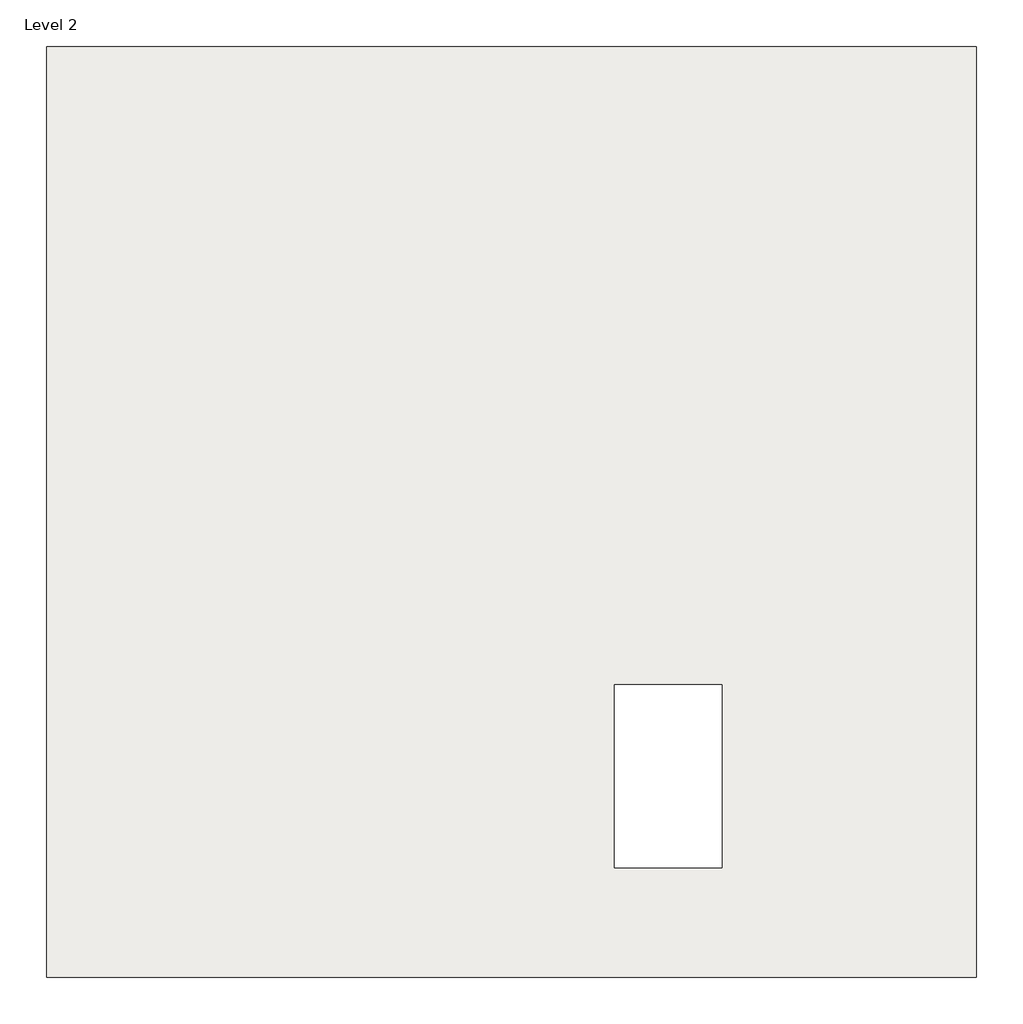
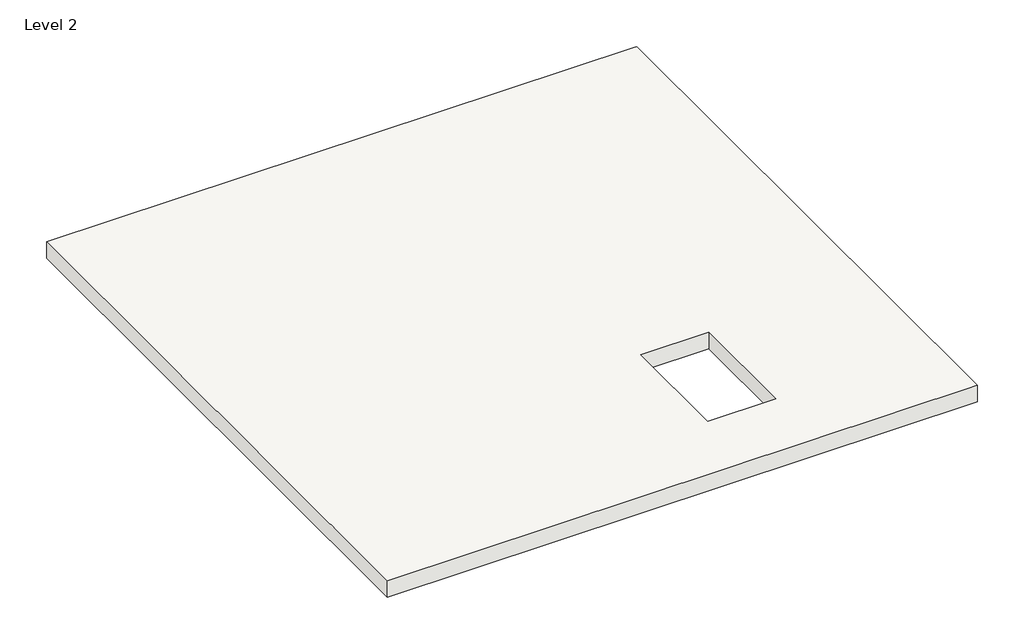
# One storey: 1 roof.
"""IFC4 building model written with IfcOpenShell, lengths in millimetres."""

from ifc_helpers import new_model, si_unit, frame, origin, place, context, project, spatial, polyline, outline, extrude, element, save

model = new_model("IFC4")

# Units and contexts
model_context = context("Model", 3, world=origin())
ifc_project = project(units=[si_unit("LENGTHUNIT", "METRE", prefix="MILLI")], contexts=[model_context])

# Site, building, storey
site = spatial("IfcSite", under=ifc_project)
building = spatial("IfcBuilding", under=site)
storey = spatial("IfcBuildingStorey", under=building, Name="Level 2", Elevation=3048.0)

# Roof
placement = place(None, origin())
element("IfcRoof", 1, ObjectType="Steel Truss - Insulation on Metal Deck - EPDM", at=placement, inside=storey, context=model_context, shape_type="SweptSolid", body=[
    extrude(outline(polyline([(-7877.0402326, 14000.8633056), (10541.1347674, 14000.8633056), (10601.4597674, 14000.8633056), (10601.4597674, -4490.3366944), (-7877.0402326, -4490.3366944), (-7877.0402326, 14000.8633056)]), holes=[polyline([(5546.8597674, 1325.1758265), (3413.2597674, 1325.1758265), (3413.2597674, -2307.0241735), (5445.2597674, -2307.0241735), (5546.8597674, -2307.0241735), (5546.8597674, 1325.1758265)])]), frame((0.0, 0.0, 3048.0), z_axis=(0.0, 0.0, 1.0), x_axis=(1.0, 0.0, 0.0)), (0.0, 0.0, 1.0), 546.1),
])

save(model, "model.ifc")

# Revit data of these elements
# Type "Steel Truss - Insulation on Metal Deck - EPDM"
#   Assembly Code = "B1020"
#   Layers, outside or top first: 0' - 0 1/4" "Roofing, EPDM Membrane" (function 4); 0' - 5" "Rigid insulation" (function 3); 0' - 0 1/4" "Metal Deck" (function 1); 1' - 4" "Structure, Steel Bar Joist Layer" (function 1)
# Element 1 (IfcRoof, "Steel Truss - Insulation on Metal Deck - EPDM")
#   built-in parameter 1001705 = 11.7917 (stored number, unit not read)
#   built-in parameter 1001710 = 33615
#   Phase Created = New Construction
#   Materials on its faces: "Structure, Steel Bar Joist Layer", "Roofing, EPDM Membrane"
# Materials
#   "Roofing, EPDM Membrane": class "Generic", colour RGB 127 127 127, transparency 0, Description = "EPDM roof membrane", Cost = 0
#   "Rigid insulation": class "Generic", colour RGB 127 127 127, transparency 0, Description = "Rigid foam insulation board", Cost = 0
#   "Metal Deck": class "Metal", colour RGB 199 199 199, transparency 0, Description = "Steel, mill finish", Cost = 0
#   "Structure, Steel Bar Joist Layer": class "Metal", colour RGB 127 127 127, transparency 0, Description = "Bar joists, thermal airspace", Cost = 0
